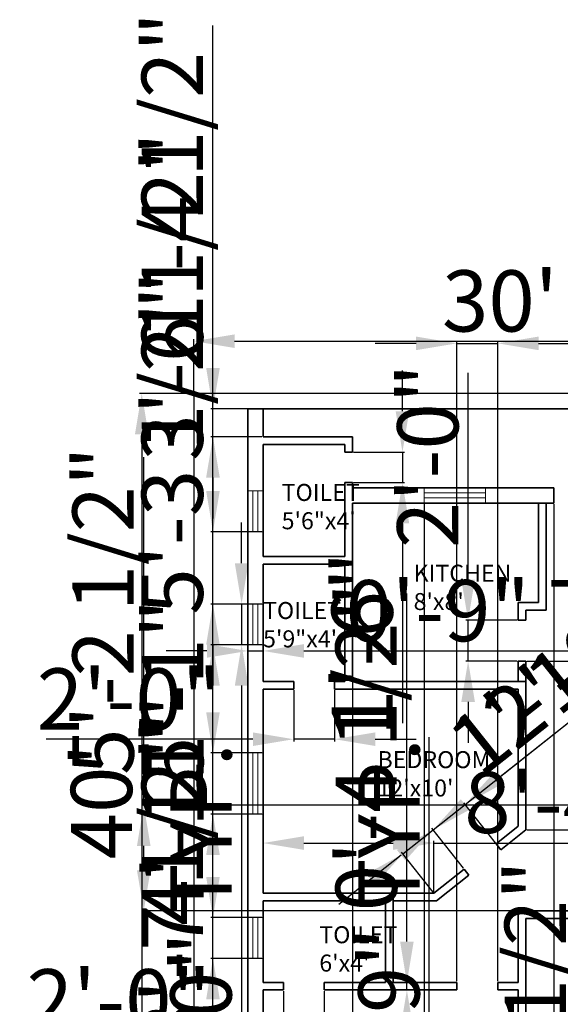
# Model space of a CAD drawing. Units: inches. Extents: x 1041 to 1781, y -140 to 732.
# Tile 2 of 6: x 1041 to 1359, y 153 to 732. Entities that reach past the tile are written whole.
import ezdxf

# ---------------------------------------------------------------- set-up
doc = ezdxf.new("R2010")
doc.units = ezdxf.units.IN
for name, color, linetype, lineweight in [('A-AREA-IDEN', 7, 'Continuous', 20), ('A-GLAZ', 4, 'Continuous', 18), ('A-WALL', 7, 'Continuous', 35), ('C-PROP', 3, 'Continuous', 25), ('dimension', 130, 'Continuous', 18)]:
    doc.layers.add(name, color=color, linetype=linetype, lineweight=lineweight)
doc.styles.get("Standard").update_dxf_attribs({"font": 'arial.ttf'})
doc.dimstyles.new('ISO-25', dxfattribs={"dimtxt": 36, "dimasz": 24, "dimexe": 1.25, "dimexo": 0.625, "dimtad": 1, "dimlunit": 4, "dimtxsty": 'Standard', "dimcen": 2.5, "dimadec": 0, "dimazin": 0, "dimtfac": 1, "dimtmove": 0, "dimatfit": 3, "dimfxl": 1, "dimarcsym": 0})

# ---------------------------------------------------------------- blocks, each defined once
blk = doc.blocks.new('*D1')
at = {"layer": 'Defpoints', "color": 0, "transparency": 16777216}
for p in [(1503.25, 542.96), (1143.25, 512.23), (1503.25, 512.23)]:
    blk.add_point(p, dxfattribs=at)
at = {"layer": 'dimension', "color": 0, "lineweight": -2, "transparency": 16777216}
for p, q in [((1143.25, 512.86), (1143.25, 544.21)), ((1167.25, 542.96), (1479.25, 542.96)), ((1503.25, 512.86), (1503.25, 544.21))]:
    blk.add_line(p, q, dxfattribs=at)
at = {"layer": 'dimension', "color": 0, "transparency": 16777216}
for points in [[(1167.25, 546.96), (1167.25, 538.96), (1143.25, 542.96)], [(1479.25, 546.96), (1479.25, 538.96), (1503.25, 542.96)]]:
    blk.add_solid(points, dxfattribs=at)
at = {"layer": 'dimension', "color": 0, "transparency": 16777216, "insert": (1323.25, 561.98), "char_height": 36, "attachment_point": 5}
blk.add_mtext("30'", dxfattribs=at)
blk = doc.blocks.new('*D2')
at = {"layer": 'Defpoints', "color": 0, "transparency": 16777216}
for p in [(1143.25, 512.23), (1112.63, 32.23), (1143.25, 32.23)]:
    blk.add_point(p, dxfattribs=at)
at = {"layer": 'dimension', "color": 0, "lineweight": -2, "transparency": 16777216}
for p, q in [((1142.62, 512.23), (1111.38, 512.23)), ((1112.63, 488.23), (1112.63, 56.23)), ((1142.62, 32.23), (1111.38, 32.23))]:
    blk.add_line(p, q, dxfattribs=at)
at = {"layer": 'dimension', "color": 0, "transparency": 16777216}
for points in [[(1108.63, 488.23), (1116.63, 488.23), (1112.63, 512.23)], [(1108.63, 56.23), (1116.63, 56.23), (1112.63, 32.23)]]:
    blk.add_solid(points, dxfattribs=at)
at = {"layer": 'dimension', "color": 0, "transparency": 16777216, "insert": (1093.62, 272.23), "char_height": 36, "attachment_point": 5, "rotation": 90}
blk.add_mtext("40'", dxfattribs=at)
blk = doc.blocks.new('WIN-36IN')
for p, q in [((0, 9), (0, 0)), ((36, 9), (0, 9)), ((36, 6), (0, 6)), ((36, 0), (36, 9)), ((0, 3), (36, 3)), ((0, 0), (36, 0)), ((0, 0), (36, 0))]:
    blk.add_line(p, q)
blk = doc.blocks.new('WIN-24IN')
for p, q in [((0, 9), (24, 9)), ((24, 9), (0, 9)), ((0, 9), (0, 0)), ((24, 6), (0, 6)), ((24, 0), (24, 9)), ((0, 3), (24, 3)), ((0, 0), (24, 0))]:
    blk.add_line(p, q)
blk = doc.blocks.new('*D9')
at = {"layer": 'Defpoints', "color": 0, "transparency": 16777216}
for p in [(1174.94, 388.32), (1171.34, 364.32), (1174.94, 364.32)]:
    blk.add_point(p, dxfattribs=at)
at = {"layer": 'dimension', "color": 0, "lineweight": -2, "transparency": 16777216}
for p, q in [((1171.34, 412.32), (1171.34, 436.32)), ((1174.31, 388.32), (1170.09, 388.32)), ((1171.34, 388.32), (1171.34, 364.32)), ((1174.31, 364.32), (1170.09, 364.32)), ((1171.34, 340.32), (1171.34, -140.48))]:
    blk.add_line(p, q, dxfattribs=at)
at = {"layer": 'dimension', "color": 0, "transparency": 16777216}
for points in [[(1167.34, 412.32), (1175.34, 412.32), (1171.34, 388.32)], [(1167.34, 340.32), (1175.34, 340.32), (1171.34, 364.32)]]:
    blk.add_solid(points, dxfattribs=at)
at = {"layer": 'dimension', "color": 0, "transparency": 16777216, "insert": (1152.09, 87.92), "char_height": 36, "attachment_point": 5, "rotation": 90}
blk.add_mtext('WINDOW 2\'-0" TYP.', dxfattribs=at)
blk = doc.blocks.new('*D10')
at = {"layer": 'Defpoints', "color": 0, "transparency": 16777216}
for p in [(1174.94, 364.32), (1183.94, 364.32), (1183.94, 360.72)]:
    blk.add_point(p, dxfattribs=at)
at = {"layer": 'dimension', "color": 0, "lineweight": -2, "transparency": 16777216}
for p, q in [((1150.94, 360.72), (1126.94, 360.72)), ((1174.94, 363.69), (1174.94, 359.47)), ((1174.94, 360.72), (1183.94, 360.72)), ((1183.94, 363.69), (1183.94, 359.47)), ((1207.94, 360.72), (1452.63, 360.72))]:
    blk.add_line(p, q, dxfattribs=at)
at = {"layer": 'dimension', "color": 0, "transparency": 16777216}
for points in [[(1150.94, 364.72), (1150.94, 356.72), (1174.94, 360.72)], [(1207.94, 364.72), (1207.94, 356.72), (1183.94, 360.72)]]:
    blk.add_solid(points, dxfattribs=at)
at = {"layer": 'dimension', "color": 0, "transparency": 16777216, "insert": (1342.28, 379.72), "char_height": 36, "attachment_point": 5}
blk.add_mtext('0\'-9" TYP.', dxfattribs=at)
blk = doc.blocks.new('*D12')
at = {"layer": 'Defpoints', "color": 0, "transparency": 16777216}
for p in [(1276.2, 41.23), (1281.6, 41.23), (1276.2, 32.23)]:
    blk.add_point(p, dxfattribs=at)
at = {"layer": 'dimension', "color": 0, "lineweight": -2, "transparency": 16777216}
for p, q in [((1281.6, 65.23), (1281.6, 309.92)), ((1276.83, 41.23), (1282.85, 41.23)), ((1281.6, 32.23), (1281.6, 41.23)), ((1276.83, 32.23), (1282.85, 32.23)), ((1281.6, 8.23), (1281.6, -15.77))]:
    blk.add_line(p, q, dxfattribs=at)
at = {"layer": 'dimension', "color": 0, "transparency": 16777216}
for points in [[(1277.6, 65.23), (1285.6, 65.23), (1281.6, 41.23)], [(1277.6, 8.23), (1285.6, 8.23), (1281.6, 32.23)]]:
    blk.add_solid(points, dxfattribs=at)
at = {"layer": 'dimension', "color": 0, "transparency": 16777216, "insert": (1262.59, 199.58), "char_height": 36, "attachment_point": 5, "rotation": 90}
blk.add_mtext('0\'-9" TYP.', dxfattribs=at)
blk = doc.blocks.new('*D19')
at = {"layer": 'Defpoints', "color": 0, "transparency": 16777216}
for p in [(1354.94, 447.73), (1390.94, 447.73), (1390.94, 2.78)]:
    blk.add_point(p, dxfattribs=at)
at = {"layer": 'dimension', "color": 0, "lineweight": -2, "transparency": 16777216}
for p, q in [((1354.94, 447.11), (1354.94, 1.53)), ((1390.94, 447.11), (1390.94, 1.53)), ((1330.94, 2.78), (1306.94, 2.78)), ((1354.94, 2.78), (1390.94, 2.78)), ((1414.94, 2.78), (1535.86, 2.78))]:
    blk.add_line(p, q, dxfattribs=at)
at = {"layer": 'dimension', "color": 0, "transparency": 16777216}
for points in [[(1330.94, 6.78), (1330.94, -1.22), (1354.94, 2.78)], [(1414.94, 6.78), (1414.94, -1.22), (1390.94, 2.78)]]:
    blk.add_solid(points, dxfattribs=at)
at = {"layer": 'dimension', "color": 0, "transparency": 16777216, "insert": (1487.4, 21.8), "char_height": 36, "attachment_point": 5}
blk.add_mtext('3\'-0"', dxfattribs=at)
blk = doc.blocks.new('*D23')
at = {"layer": 'Defpoints', "color": 0, "transparency": 16777216}
for p in [(1302.68, 270.36), (1321, 247.3), (1302.2, 232.37)]:
    blk.add_point(p, dxfattribs=at)
at = {"layer": 'dimension', "color": 0, "lineweight": -2, "transparency": 16777216}
for p, q in [((1321.47, 285.29), (1416.66, 360.9)), ((1283.89, 255.44), (1302.68, 270.36)), ((1320.61, 247.79), (1301.9, 271.34)), ((1301.82, 232.86), (1283.11, 256.41)), ((1265.09, 240.51), (1246.3, 225.58))]:
    blk.add_line(p, q, dxfattribs=at)
at = {"layer": 'dimension', "color": 0, "transparency": 16777216}
for points in [[(1318.99, 288.42), (1323.96, 282.16), (1302.68, 270.36)], [(1262.61, 243.64), (1267.58, 237.38), (1283.89, 255.44)]]:
    blk.add_solid(points, dxfattribs=at)
at = {"layer": 'dimension', "color": 0, "transparency": 16777216, "insert": (1366.64, 345.44), "char_height": 36, "attachment_point": 5, "rotation": 38.45936}
blk.add_mtext('2\'-0"', dxfattribs=at)
blk = doc.blocks.new('*D24')
at = {"layer": 'Defpoints', "color": 0, "transparency": 16777216}
for p in [(1154.49, 84.57), (1183.94, 84.57), (1183.94, 41.23)]:
    blk.add_point(p, dxfattribs=at)
at = {"layer": 'dimension', "color": 0, "lineweight": -2, "transparency": 16777216}
for p, q in [((1154.49, 108.57), (1154.49, 313.38)), ((1183.31, 84.57), (1153.24, 84.57)), ((1154.49, 41.23), (1154.49, 84.57)), ((1183.31, 41.23), (1153.24, 41.23)), ((1154.49, 17.23), (1154.49, -6.77))]:
    blk.add_line(p, q, dxfattribs=at)
at = {"layer": 'dimension', "color": 0, "transparency": 16777216}
for points in [[(1150.49, 108.57), (1158.49, 108.57), (1154.49, 84.57)], [(1150.49, 17.23), (1158.49, 17.23), (1154.49, 41.23)]]:
    blk.add_solid(points, dxfattribs=at)
at = {"layer": 'dimension', "color": 0, "transparency": 16777216, "insert": (1135.24, 222.98), "char_height": 36, "attachment_point": 5, "rotation": 90}
blk.add_mtext('3\'-7 1/2"', dxfattribs=at)
blk = doc.blocks.new('*D25')
at = {"layer": 'Defpoints', "color": 0, "transparency": 16777216}
for p in [(1154.49, 179.79), (1183.94, 179.79), (1183.94, 120.57)]:
    blk.add_point(p, dxfattribs=at)
at = {"layer": 'dimension', "color": 0, "lineweight": -2, "transparency": 16777216}
for p, q in [((1154.49, 179.79), (1154.49, 330.15)), ((1183.31, 179.79), (1153.24, 179.79)), ((1154.49, 144.57), (1154.49, 155.79)), ((1183.31, 120.57), (1153.24, 120.57))]:
    blk.add_line(p, q, dxfattribs=at)
at = {"layer": 'dimension', "color": 0, "transparency": 16777216}
for points in [[(1150.49, 155.79), (1158.49, 155.79), (1154.49, 179.79)], [(1150.49, 144.57), (1158.49, 144.57), (1154.49, 120.57)]]:
    blk.add_solid(points, dxfattribs=at)
at = {"layer": 'dimension', "color": 0, "transparency": 16777216, "insert": (1135.79, 266.97), "char_height": 36, "attachment_point": 5, "rotation": 90}
blk.add_mtext('4\'-11"', dxfattribs=at)
blk = doc.blocks.new('*D26')
at = {"layer": 'Defpoints', "color": 0, "transparency": 16777216}
for p in [(1154.49, 264.67), (1183.94, 264.67), (1183.94, 203.79)]:
    blk.add_point(p, dxfattribs=at)
at = {"layer": 'dimension', "color": 0, "lineweight": -2, "transparency": 16777216}
for p, q in [((1154.49, 264.67), (1154.49, 385.62)), ((1183.31, 264.67), (1153.24, 264.67)), ((1154.49, 227.79), (1154.49, 240.67)), ((1183.31, 203.79), (1153.24, 203.79))]:
    blk.add_line(p, q, dxfattribs=at)
at = {"layer": 'dimension', "color": 0, "transparency": 16777216}
for points in [[(1150.49, 240.67), (1158.49, 240.67), (1154.49, 264.67)], [(1150.49, 227.79), (1158.49, 227.79), (1154.49, 203.79)]]:
    blk.add_solid(points, dxfattribs=at)
at = {"layer": 'dimension', "color": 0, "transparency": 16777216, "insert": (1135.48, 337.15), "char_height": 36, "attachment_point": 5, "rotation": 90}
blk.add_mtext('5\'-1"', dxfattribs=at)
blk = doc.blocks.new('*D27')
at = {"layer": 'Defpoints', "color": 0, "transparency": 16777216}
for p in [(1154.49, 364.32), (1183.94, 364.32), (1183.94, 300.67)]:
    blk.add_point(p, dxfattribs=at)
at = {"layer": 'dimension', "color": 0, "lineweight": -2, "transparency": 16777216}
for p, q in [((1154.49, 364.32), (1154.49, 569.15)), ((1183.31, 364.32), (1153.24, 364.32)), ((1154.49, 324.67), (1154.49, 340.32)), ((1183.31, 300.67), (1153.24, 300.67))]:
    blk.add_line(p, q, dxfattribs=at)
at = {"layer": 'dimension', "color": 0, "transparency": 16777216}
for points in [[(1150.49, 340.32), (1158.49, 340.32), (1154.49, 364.32)], [(1150.49, 324.67), (1158.49, 324.67), (1154.49, 300.67)]]:
    blk.add_solid(points, dxfattribs=at)
at = {"layer": 'dimension', "color": 0, "transparency": 16777216, "insert": (1135.24, 478.73), "char_height": 36, "attachment_point": 5, "rotation": 90}
blk.add_mtext('5\'-3 1/2"', dxfattribs=at)
blk = doc.blocks.new('*D28')
at = {"layer": 'Defpoints', "color": 0, "transparency": 16777216}
for p in [(1154.49, 430.87), (1183.94, 430.87), (1183.94, 388.32)]:
    blk.add_point(p, dxfattribs=at)
at = {"layer": 'dimension', "color": 0, "lineweight": -2, "transparency": 16777216}
for p, q in [((1154.49, 454.87), (1154.49, 659.68)), ((1183.31, 430.87), (1153.24, 430.87)), ((1154.49, 388.32), (1154.49, 430.87)), ((1183.31, 388.32), (1153.24, 388.32)), ((1154.49, 364.32), (1154.49, 340.32))]:
    blk.add_line(p, q, dxfattribs=at)
at = {"layer": 'dimension', "color": 0, "transparency": 16777216}
for points in [[(1150.49, 454.87), (1158.49, 454.87), (1154.49, 430.87)], [(1150.49, 364.32), (1158.49, 364.32), (1154.49, 388.32)]]:
    blk.add_solid(points, dxfattribs=at)
at = {"layer": 'dimension', "color": 0, "transparency": 16777216, "insert": (1135.24, 569.28), "char_height": 36, "attachment_point": 5, "rotation": 90}
blk.add_mtext('3\'-6 1/2"', dxfattribs=at)
blk = doc.blocks.new('*D29')
at = {"layer": 'Defpoints', "color": 0, "transparency": 16777216}
for p in [(1113.8, 269.99), (1467.44, 269.99), (1467.44, 207.73)]:
    blk.add_point(p, dxfattribs=at)
at = {"layer": 'dimension', "color": 0, "lineweight": -2, "transparency": 16777216}
for p, q in [((1113.8, 269.99), (1113.8, 474.82)), ((1466.81, 269.99), (1112.55, 269.99)), ((1113.8, 231.73), (1113.8, 245.99)), ((1466.81, 207.73), (1112.55, 207.73))]:
    blk.add_line(p, q, dxfattribs=at)
at = {"layer": 'dimension', "color": 0, "transparency": 16777216}
for points in [[(1109.8, 245.99), (1117.8, 245.99), (1113.8, 269.99)], [(1109.8, 231.73), (1117.8, 231.73), (1113.8, 207.73)]]:
    blk.add_solid(points, dxfattribs=at)
at = {"layer": 'dimension', "color": 0, "transparency": 16777216, "insert": (1094.56, 384.41), "char_height": 36, "attachment_point": 5, "rotation": 90}
blk.add_mtext('5\'-2 1/2"', dxfattribs=at)
blk = doc.blocks.new('*D31')
at = {"layer": 'Defpoints', "color": 0, "transparency": 16777216}
for p in [(1390.94, 447.73), (1427, 447.73), (1427, 2.78)]:
    blk.add_point(p, dxfattribs=at)
at = {"layer": 'dimension', "color": 0, "lineweight": -2, "transparency": 16777216}
for p, q in [((1390.94, 447.11), (1390.94, 1.53)), ((1427, 447.11), (1427, 1.53)), ((1366.94, 2.78), (1342.94, 2.78)), ((1390.94, 2.78), (1427, 2.78)), ((1451, 2.78), (1571.93, 2.78))]:
    blk.add_line(p, q, dxfattribs=at)
at = {"layer": 'dimension', "color": 0, "transparency": 16777216}
for points in [[(1366.94, 6.78), (1366.94, -1.22), (1390.94, 2.78)], [(1451, 6.78), (1451, -1.22), (1427, 2.78)]]:
    blk.add_solid(points, dxfattribs=at)
at = {"layer": 'dimension', "color": 0, "transparency": 16777216, "insert": (1523.46, 21.8), "char_height": 36, "attachment_point": 5}
blk.add_mtext('3\'-0"', dxfattribs=at)
blk = doc.blocks.new('*D32')
at = {"layer": 'Defpoints', "color": 0, "transparency": 16777216}
for p in [(1236.44, 447.73), (1278.74, 447.73), (1278.74, 2.78)]:
    blk.add_point(p, dxfattribs=at)
at = {"layer": 'dimension', "color": 0, "lineweight": -2, "transparency": 16777216}
for p, q in [((1236.44, 447.11), (1236.44, 1.53)), ((1278.74, 447.11), (1278.74, 1.53)), ((1212.44, 2.78), (1188.44, 2.78)), ((1236.44, 2.78), (1278.74, 2.78)), ((1302.74, 2.78), (1507.55, 2.78))]:
    blk.add_line(p, q, dxfattribs=at)
at = {"layer": 'dimension', "color": 0, "transparency": 16777216}
for points in [[(1212.44, 6.78), (1212.44, -1.22), (1236.44, 2.78)], [(1302.74, 6.78), (1302.74, -1.22), (1278.74, 2.78)]]:
    blk.add_solid(points, dxfattribs=at)
at = {"layer": 'dimension', "color": 0, "transparency": 16777216, "insert": (1417.15, 22.03), "char_height": 36, "attachment_point": 5}
blk.add_mtext('3\'-6 1/2"', dxfattribs=at)
blk = doc.blocks.new('*D34')
at = {"layer": 'Defpoints', "color": 0, "transparency": 16777216}
for p in [(1236.44, 477.73), (1236.44, 459.73), (1265.89, 459.73)]:
    blk.add_point(p, dxfattribs=at)
at = {"layer": 'dimension', "color": 0, "lineweight": -2, "transparency": 16777216}
for p, q in [((1265.89, 501.73), (1265.89, 525.73)), ((1237.06, 477.73), (1267.14, 477.73)), ((1265.89, 477.73), (1265.89, 459.73)), ((1237.06, 459.73), (1267.14, 459.73)), ((1265.89, 435.73), (1265.89, 318.17))]:
    blk.add_line(p, q, dxfattribs=at)
at = {"layer": 'dimension', "color": 0, "transparency": 16777216}
for points in [[(1261.89, 501.73), (1269.89, 501.73), (1265.89, 477.73)], [(1261.89, 435.73), (1269.89, 435.73), (1265.89, 459.73)]]:
    blk.add_solid(points, dxfattribs=at)
at = {"layer": 'dimension', "color": 0, "transparency": 16777216, "insert": (1246.88, 364.95), "char_height": 36, "attachment_point": 5, "rotation": 90}
blk.add_mtext('1\'-6"', dxfattribs=at)
blk = doc.blocks.new('*D35')
at = {"layer": 'Defpoints', "color": 0, "transparency": 16777216}
for p in [(1321.94, 541.68), (1297.94, 165.73), (1321.94, 165.73)]:
    blk.add_point(p, dxfattribs=at)
at = {"layer": 'dimension', "color": 0, "lineweight": -2, "transparency": 16777216}
for p, q in [((1273.94, 541.68), (1249.94, 541.68)), ((1297.94, 166.36), (1297.94, 542.93)), ((1297.94, 541.68), (1321.94, 541.68)), ((1321.94, 166.36), (1321.94, 542.93)), ((1345.94, 541.68), (1467.5, 541.68))]:
    blk.add_line(p, q, dxfattribs=at)
at = {"layer": 'dimension', "color": 0, "transparency": 16777216}
for points in [[(1273.94, 545.68), (1273.94, 537.68), (1297.94, 541.68)], [(1345.94, 545.68), (1345.94, 537.68), (1321.94, 541.68)]]:
    blk.add_solid(points, dxfattribs=at)
at = {"layer": 'dimension', "color": 0, "transparency": 16777216, "insert": (1418.72, 560.69), "char_height": 36, "attachment_point": 5}
blk.add_mtext('2\'-0"', dxfattribs=at)
blk = doc.blocks.new('*D36')
at = {"layer": 'Defpoints', "color": 0, "transparency": 16777216}
for p in [(1195.94, 161.23), (1219.94, 161.23), (1195.94, 131.78)]:
    blk.add_point(p, dxfattribs=at)
at = {"layer": 'dimension', "color": 0, "lineweight": -2, "transparency": 16777216}
for p, q in [((1195.94, 160.61), (1195.94, 130.53)), ((1219.94, 160.61), (1219.94, 130.53)), ((1171.94, 131.78), (1050.38, 131.78)), ((1219.94, 131.78), (1195.94, 131.78)), ((1243.94, 131.78), (1267.94, 131.78))]:
    blk.add_line(p, q, dxfattribs=at)
at = {"layer": 'dimension', "color": 0, "transparency": 16777216}
for points in [[(1171.94, 135.78), (1171.94, 127.78), (1195.94, 131.78)], [(1243.94, 135.78), (1243.94, 127.78), (1219.94, 131.78)]]:
    blk.add_solid(points, dxfattribs=at)
at = {"layer": 'dimension', "color": 0, "transparency": 16777216, "insert": (1099.16, 150.79), "char_height": 36, "attachment_point": 5}
blk.add_mtext('2\'-0"', dxfattribs=at)
blk = doc.blocks.new('*D37')
at = {"layer": 'Defpoints', "color": 0, "transparency": 16777216}
for p in [(1201.94, 338.23), (1225.94, 338.23), (1201.94, 308.78)]:
    blk.add_point(p, dxfattribs=at)
at = {"layer": 'dimension', "color": 0, "lineweight": -2, "transparency": 16777216}
for p, q in [((1201.94, 337.61), (1201.94, 307.53)), ((1225.94, 337.61), (1225.94, 307.53)), ((1177.94, 308.78), (1056.38, 308.78)), ((1225.94, 308.78), (1201.94, 308.78)), ((1249.94, 308.78), (1273.94, 308.78))]:
    blk.add_line(p, q, dxfattribs=at)
at = {"layer": 'dimension', "color": 0, "transparency": 16777216}
for points in [[(1177.94, 312.78), (1177.94, 304.78), (1201.94, 308.78)], [(1249.94, 312.78), (1249.94, 304.78), (1225.94, 308.78)]]:
    blk.add_solid(points, dxfattribs=at)
at = {"layer": 'dimension', "color": 0, "transparency": 16777216, "insert": (1105.16, 327.79), "char_height": 36, "attachment_point": 5}
blk.add_mtext('2\'-0"', dxfattribs=at)
blk = doc.blocks.new('*D38')
at = {"layer": 'Defpoints', "color": 0, "transparency": 16777216}
for p in [(1304.49, 378.73), (1333.94, 378.73), (1333.94, 354.73)]:
    blk.add_point(p, dxfattribs=at)
at = {"layer": 'dimension', "color": 0, "lineweight": -2, "transparency": 16777216}
for p, q in [((1304.49, 402.73), (1304.49, 524.29)), ((1333.31, 378.73), (1303.24, 378.73)), ((1304.49, 354.73), (1304.49, 378.73)), ((1333.31, 354.73), (1303.24, 354.73)), ((1304.49, 330.73), (1304.49, 306.73))]:
    blk.add_line(p, q, dxfattribs=at)
at = {"layer": 'dimension', "color": 0, "transparency": 16777216}
for points in [[(1300.49, 402.73), (1308.49, 402.73), (1304.49, 378.73)], [(1300.49, 330.73), (1308.49, 330.73), (1304.49, 354.73)]]:
    blk.add_solid(points, dxfattribs=at)
at = {"layer": 'dimension', "color": 0, "transparency": 16777216, "insert": (1285.48, 475.51), "char_height": 36, "attachment_point": 5, "rotation": 90}
blk.add_mtext('2\'-0"', dxfattribs=at)
blk = doc.blocks.new('*D40')
at = {"layer": 'Defpoints', "color": 0, "transparency": 16777216}
for p in [(1154.49, 503.23), (1183.94, 503.23), (1183.94, 486.73)]:
    blk.add_point(p, dxfattribs=at)
at = {"layer": 'dimension', "color": 0, "lineweight": -2, "transparency": 16777216}
for p, q in [((1154.49, 527.23), (1154.49, 728.68)), ((1183.31, 503.23), (1153.24, 503.23)), ((1154.49, 486.73), (1154.49, 503.23)), ((1183.31, 486.73), (1153.24, 486.73)), ((1154.49, 462.73), (1154.49, 438.73))]:
    blk.add_line(p, q, dxfattribs=at)
at = {"layer": 'dimension', "color": 0, "transparency": 16777216}
for points in [[(1150.49, 527.23), (1158.49, 527.23), (1154.49, 503.23)], [(1150.49, 462.73), (1158.49, 462.73), (1154.49, 486.73)]]:
    blk.add_solid(points, dxfattribs=at)
at = {"layer": 'dimension', "color": 0, "transparency": 16777216, "insert": (1135.25, 639.95), "char_height": 36, "attachment_point": 5, "rotation": 90}
blk.add_mtext('1\'-4 1/2"', dxfattribs=at)
blk = doc.blocks.new('*D41')
at = {"layer": 'Defpoints', "color": 0, "transparency": 16777216}
for p in [(1268.49, 165.73), (1297.94, 165.73), (1297.94, 161.23)]:
    blk.add_point(p, dxfattribs=at)
at = {"layer": 'dimension', "color": 0, "lineweight": -2, "transparency": 16777216}
for p, q in [((1268.49, 189.73), (1268.49, 394.57)), ((1297.31, 165.73), (1267.24, 165.73)), ((1268.49, 161.23), (1268.49, 165.73)), ((1297.31, 161.23), (1267.24, 161.23)), ((1268.49, 137.23), (1268.49, 113.23))]:
    blk.add_line(p, q, dxfattribs=at)
at = {"layer": 'dimension', "color": 0, "transparency": 16777216}
for points in [[(1264.49, 189.73), (1272.49, 189.73), (1268.49, 165.73)], [(1264.49, 137.23), (1272.49, 137.23), (1268.49, 161.23)]]:
    blk.add_solid(points, dxfattribs=at)
at = {"layer": 'dimension', "color": 0, "transparency": 16777216, "insert": (1249.25, 304.15), "char_height": 36, "attachment_point": 5, "rotation": 90}
blk.add_mtext('0\'-4 1/2"', dxfattribs=at)
blk = doc.blocks.new('*D43')
at = {"layer": 'Defpoints', "color": 0, "transparency": 16777216}
for p in [(1284.4, 247.68), (1183.94, 218.23), (1284.4, 218.23)]:
    blk.add_point(p, dxfattribs=at)
at = {"layer": 'dimension', "color": 0, "lineweight": -2, "transparency": 16777216}
for p, q in [((1183.94, 218.86), (1183.94, 248.93)), ((1207.94, 247.68), (1260.4, 247.68)), ((1284.4, 218.86), (1284.4, 248.93)), ((1284.4, 247.68), (1489.28, 247.68))]:
    blk.add_line(p, q, dxfattribs=at)
at = {"layer": 'dimension', "color": 0, "transparency": 16777216}
for points in [[(1207.94, 251.68), (1207.94, 243.68), (1183.94, 247.68)], [(1260.4, 251.68), (1260.4, 243.68), (1284.4, 247.68)]]:
    blk.add_solid(points, dxfattribs=at)
at = {"layer": 'dimension', "color": 0, "transparency": 16777216, "insert": (1398.84, 266.92), "char_height": 36, "attachment_point": 5}
blk.add_mtext('8\'-4 1/2"', dxfattribs=at)
blk = doc.blocks.new('*D44')
at = {"layer": 'Defpoints', "color": 0, "transparency": 16777216}
for p in [(1338.44, 354.73), (1338.44, 255.41), (1367.89, 255.41)]:
    blk.add_point(p, dxfattribs=at)
at = {"layer": 'dimension', "color": 0, "lineweight": -2, "transparency": 16777216}
for p, q in [((1339.06, 354.73), (1369.14, 354.73)), ((1367.89, 330.73), (1367.89, 279.41)), ((1339.06, 255.41), (1369.14, 255.41)), ((1367.89, 255.41), (1367.89, 50.53))]:
    blk.add_line(p, q, dxfattribs=at)
at = {"layer": 'dimension', "color": 0, "transparency": 16777216}
for points in [[(1363.89, 330.73), (1371.89, 330.73), (1367.89, 354.73)], [(1363.89, 279.41), (1371.89, 279.41), (1367.89, 255.41)]]:
    blk.add_solid(points, dxfattribs=at)
at = {"layer": 'dimension', "color": 0, "transparency": 16777216, "insert": (1348.64, 140.97), "char_height": 36, "attachment_point": 5, "rotation": 90}
blk.add_mtext('8\'-3 1/2"', dxfattribs=at)
blk = doc.blocks.new('*D45')
at = {"layer": 'Defpoints', "color": 0, "transparency": 16777216}
for p in [(1283.89, 255.44), (1302.2, 232.37), (1284.4, 218.23)]:
    blk.add_point(p, dxfattribs=at)
at = {"layer": 'dimension', "color": 0, "lineweight": -2, "transparency": 16777216}
for p, q in [((1302.68, 270.36), (1482.32, 413.05)), ((1266.08, 241.29), (1283.89, 255.44)), ((1301.82, 232.86), (1283.11, 256.41)), ((1284.01, 218.72), (1265.3, 242.27)), ((1247.29, 226.37), (1228.5, 211.44))]:
    blk.add_line(p, q, dxfattribs=at)
at = {"layer": 'dimension', "color": 0, "transparency": 16777216}
for points in [[(1300.19, 273.49), (1305.17, 267.23), (1283.89, 255.44)], [(1244.8, 229.5), (1249.78, 223.23), (1266.08, 241.29)]]:
    blk.add_solid(points, dxfattribs=at)
at = {"layer": 'dimension', "color": 0, "transparency": 16777216, "insert": (1389.93, 364.23), "char_height": 36, "attachment_point": 5, "rotation": 38.45936}
blk.add_mtext('1\'-10 1/2"', dxfattribs=at)

msp = doc.modelspace()

# ---------------------------------------------------------------- linework, layer by layer
at = {"layer": 'A-GLAZ'}
for p, q in [((1278.743, 456.733), (1278.743, 447.733)), ((1278.743, 456.733), (1314.743, 456.733)), ((1314.743, 453.733), (1278.743, 453.733)), ((1314.743, 447.733), (1314.743, 456.733)), ((1278.743, 450.733), (1314.743, 450.733)), ((1278.743, 447.733), (1314.743, 447.733))]:
    msp.add_line(p, q, dxfattribs=at)
at = {"layer": 'A-WALL'}
for p, q in [((1498.749, 503.233), (1174.938, 503.233)), ((1174.938, 41.233), (1174.938, 503.233)), ((1183.938, 486.733), (1183.938, 503.233)), ((1183.938, 486.733), (1236.438, 486.733)), ((1231.938, 486.733), (1236.438, 486.733)), ((1236.438, 477.733), (1236.438, 486.733)), ((1183.938, 482.233), (1231.938, 482.233)), ((1183.938, 416.233), (1183.938, 482.233)), ((1231.938, 477.733), (1231.938, 482.233)), ((1231.938, 477.733), (1236.438, 477.733)), ((1231.938, 416.233), (1231.938, 459.733)), ((1231.938, 459.733), (1236.438, 459.733)), ((1236.438, 456.733), (1236.438, 459.733)), ((1236.438, 456.733), (1354.938, 456.733)), ((1354.938, 447.733), (1354.938, 456.733)), ((1236.438, 447.733), (1354.938, 447.733)), ((1236.438, 342.733), (1236.438, 447.733)), ((1345.938, 389.233), (1345.938, 447.733)), ((1350.438, 384.733), (1350.438, 447.733)), ((1183.938, 416.233), (1231.938, 416.233)), ((1183.938, 411.733), (1231.938, 411.733)), ((1183.938, 342.733), (1183.938, 411.733)), ((1231.938, 342.733), (1231.938, 411.733)), ((1333.938, 378.733), (1333.938, 389.233)), ((1333.938, 389.233), (1345.938, 389.233)), ((1338.438, 378.733), (1338.438, 384.733)), ((1338.438, 384.733), (1350.438, 384.733)), ((1333.938, 378.733), (1338.438, 378.733)), ((1333.938, 342.733), (1333.938, 354.733)), ((1333.938, 354.733), (1338.438, 354.733)), ((1338.438, 255.408), (1338.438, 354.733)), ((1183.938, 342.733), (1201.938, 342.733)), ((1201.938, 338.233), (1201.938, 342.733)), ((1225.938, 338.233), (1225.938, 342.733)), ((1225.938, 342.733), (1231.938, 342.733)), ((1236.438, 342.733), (1338.438, 342.733)), ((1183.938, 338.233), (1201.938, 338.233)), ((1183.938, 218.233), (1183.938, 338.233)), ((1225.938, 338.233), (1333.938, 338.233)), ((1333.938, 257.58), (1333.938, 338.233)), ((1333.938, 257.58), (1320.997, 247.302)), ((1338.438, 255.408), (1323.796, 243.778)), ((1320.997, 247.302), (1323.796, 243.778)), ((1302.204, 232.375), (1284.399, 218.233)), ((1302.204, 232.375), (1305.003, 228.851)), ((1305.003, 228.851), (1285.968, 213.733)), ((1183.938, 218.233), (1284.399, 218.233)), ((1260.438, 165.733), (1260.438, 218.233)), ((1183.938, 213.733), (1255.938, 213.733)), ((1183.938, 165.733), (1183.938, 213.733)), ((1255.938, 165.733), (1255.938, 213.733)), ((1260.438, 213.733), (1285.968, 213.733)), ((1333.938, 207.733), (1413.438, 207.733)), ((1333.938, 165.733), (1333.938, 207.733)), ((1338.438, 41.233), (1338.438, 203.233)), ((1338.438, 203.233), (1413.438, 203.233)), ((1183.938, 165.733), (1195.938, 165.733)), ((1183.938, 165.733), (1195.938, 165.733)), ((1195.938, 165.733), (1195.938, 161.233)), ((1219.938, 165.733), (1219.938, 161.233)), ((1219.938, 165.733), (1255.938, 165.733)), ((1260.438, 165.733), (1297.938, 165.733)), ((1297.938, 165.733), (1297.938, 161.233)), ((1333.938, 165.733), (1321.938, 165.733)), ((1321.938, 165.733), (1321.938, 161.233)), ((1321.938, 165.733), (1333.938, 165.733)), ((1183.938, 161.233), (1195.938, 161.233)), ((1183.938, 41.233), (1183.938, 161.233)), ((1219.938, 161.233), (1297.938, 161.233)), ((1321.938, 161.233), (1333.938, 161.233)), ((1333.938, 41.233), (1333.938, 161.233))]:
    msp.add_line(p, q, dxfattribs=at)
at = {"layer": 'C-PROP'}
for p, q in [((1503.249, 512.233), (1143.249, 512.233)), ((1143.249, 512.233), (1143.249, 32.233))]:
    msp.add_line(p, q, dxfattribs=at)

# ---------------------------------------------------------------- block references
at = {"layer": 'A-GLAZ'}
for name, p, rotation in [('WIN-24IN', (1174.938, 454.873), 269.9999999999987), ('WIN-24IN', (1174.938, 388.318), 269.9999999999987), ('WIN-36IN', (1183.937, 264.674), 89.9999999999994), ('WIN-24IN', (1174.938, 203.788), 269.9999999999986)]:
    msp.add_blockref(name, p, dxfattribs=dict(at, rotation=rotation))

# ---------------------------------------------------------------- texts
at = {"layer": 'A-AREA-IDEN', "char_height": 10, "attachment_point": 1}
for s, insert in [('TOILET\\P5\'6"x4\'', (1194.873, 458.97)), ("KITCHEN\\P8'x8'", (1272.445, 411.441)), ('TOILET\\P5\'9"x4\'', (1183.938, 389.504)), ("BEDROOM\\P12'x10'", (1251.223, 301.757)), ("TOILET\\P6'x4'", (1217.009, 198.743))]:
    msp.add_mtext_dynamic_manual_height_columns(s, width=64.5482, gutter_width=12.5, heights=[0], dxfattribs=dict(at, insert=insert))

# ---------------------------------------------------------------- dimensions: what is measured, and where the dimension line sits
at = {"layer": 'dimension'}
for base, p1, p2, angle, override, picture, middle in [((1154.488, 503.233), (1183.938, 486.733), (1183.938, 503.233), 90, {"dimdec": 1, "dimlfac": 1, "dimrnd": 0, "dimzin": 1, "dimdsep": 46, "dimlunit": 4, "dimfrac": 2}, '*D40', (1135.249, 639.954)), ((1154.488, 430.873), (1183.938, 388.318), (1183.938, 430.873), 90, {"dimdec": 1, "dimlfac": 1, "dimrnd": 0, "dimzin": 1, "dimdsep": 46, "dimlunit": 4, "dimfrac": 2}, '*D28', (1135.236, 569.277)), ((1154.488, 364.318), (1183.938, 300.673), (1183.938, 364.318), 90, {"dimdec": 1, "dimlfac": 1, "dimrnd": 0, "dimzin": 1, "dimdsep": 46, "dimlunit": 4, "dimfrac": 2}, '*D27', (1135.236, 478.734)), ((1304.488, 378.733), (1333.938, 354.733), (1333.938, 378.733), 90, {"dimdec": 1, "dimlfac": 1, "dimrnd": 0, "dimzin": 1, "dimdsep": 46, "dimlunit": 4, "dimfrac": 2}, '*D38', (1285.482, 475.513)), ((1265.888, 459.733), (1236.438, 477.733), (1236.438, 459.733), 270, {"dimdec": 1, "dimlfac": 1, "dimrnd": 0, "dimzin": 1, "dimdsep": 46, "dimlunit": 4, "dimfrac": 2}, '*D34', (1246.882, 364.953)), ((1112.63, 32.233), (1143.249, 512.233), (1143.249, 32.233), 90, {"dimclrd": 0, "dimclre": 0, "dimclrt": 0}, '*D2', (1093.625, 272.233)), ((1113.799, 269.99), (1467.438, 207.733), (1467.438, 269.99), 90, {"dimdec": 1, "dimlfac": 1, "dimrnd": 0, "dimzin": 1, "dimdsep": 46, "dimlunit": 4, "dimfrac": 2}, '*D29', (1094.56, 384.406)), ((1283.887, 255.436), (1284.399, 218.233), (1302.204, 232.375), 38.459364, {"dimdec": 1, "dimlfac": 1, "dimrnd": 0, "dimzin": 1, "dimdsep": 46, "dimlunit": 4, "dimfrac": 2}, '*D45', (1389.932, 364.234)), ((1268.488, 165.733), (1297.938, 161.233), (1297.938, 165.733), 90, {"dimdec": 1, "dimlfac": 1, "dimrnd": 0, "dimzin": 1, "dimdsep": 46, "dimlunit": 4, "dimfrac": 2}, '*D41', (1249.249, 304.149)), ((1302.68, 270.363), (1302.204, 232.375), (1320.997, 247.302), 38.459364, {"dimdec": 1, "dimlfac": 1, "dimrnd": 0, "dimzin": 1, "dimdsep": 46, "dimlunit": 4, "dimfrac": 2}, '*D23', (1366.644, 345.439)), ((1154.488, 264.673), (1183.938, 203.788), (1183.938, 264.673), 90, {"dimdec": 1, "dimlfac": 1, "dimrnd": 0, "dimzin": 1, "dimdsep": 46, "dimlunit": 4, "dimfrac": 2}, '*D26', (1135.482, 337.147)), ((1367.888, 255.408), (1338.438, 354.733), (1338.438, 255.408), 270, {"dimdec": 1, "dimlfac": 1, "dimrnd": 0, "dimzin": 1, "dimdsep": 46, "dimlunit": 4, "dimfrac": 2}, '*D44', (1348.636, 140.967)), ((1201.938, 308.783), (1225.938, 338.233), (1201.938, 338.233), 180, {"dimdec": 1, "dimlfac": 1, "dimrnd": 0, "dimzin": 1, "dimdsep": 46, "dimlunit": 4, "dimfrac": 2}, '*D37', (1105.157, 327.788)), ((1154.488, 179.788), (1183.938, 120.573), (1183.938, 179.788), 90, {"dimdec": 1, "dimlfac": 1, "dimrnd": 0, "dimzin": 1, "dimdsep": 46, "dimlunit": 4, "dimfrac": 2}, '*D25', (1135.789, 266.971)), ((1154.488, 84.573), (1183.938, 41.233), (1183.938, 84.573), 90, {"dimdec": 1, "dimlfac": 1, "dimrnd": 0, "dimzin": 1, "dimdsep": 46, "dimlunit": 4, "dimfrac": 2}, '*D24', (1135.236, 222.977)), ((1195.938, 131.783), (1219.938, 161.233), (1195.938, 161.233), 180, {"dimdec": 1, "dimlfac": 1, "dimrnd": 0, "dimzin": 1, "dimdsep": 46, "dimlunit": 4, "dimfrac": 2}, '*D36', (1099.157, 150.788))]:
    dim = msp.add_linear_dim(base=base, p1=p1, p2=p2, angle=angle, dimstyle='ISO-25', override=override, dxfattribs=at)
    dim.commit()
    dim.dimension.update_dxf_attribs({"geometry": picture, "text_midpoint": middle})
for base, p1, p2, override, picture, middle in [((1503.249, 542.957), (1143.249, 512.233), (1503.249, 512.233), {"dimclrd": 0, "dimclre": 0, "dimclrt": 0}, '*D1', (1323.249, 561.975)), ((1321.938, 541.683), (1297.938, 165.733), (1321.938, 165.733), {"dimdec": 1, "dimlfac": 1, "dimrnd": 0, "dimzin": 1, "dimdsep": 46, "dimlunit": 4, "dimfrac": 2}, '*D35', (1418.718, 560.688)), ((1278.743, 2.783), (1236.438, 447.733), (1278.743, 447.733), {"dimdec": 1, "dimlfac": 1, "dimrnd": 0, "dimzin": 1, "dimdsep": 46, "dimlunit": 4, "dimfrac": 2}, '*D32', (1417.147, 22.034)), ((1390.938, 2.783), (1354.938, 447.733), (1390.938, 447.733), {"dimdec": 1, "dimlfac": 1, "dimrnd": 0, "dimzin": 1, "dimdsep": 46, "dimlunit": 4, "dimfrac": 2}, '*D19', (1487.399, 21.8)), ((1427.003, 2.783), (1390.938, 447.733), (1427.003, 447.733), {"dimdec": 1, "dimlfac": 1, "dimrnd": 0, "dimzin": 1, "dimdsep": 46, "dimlunit": 4, "dimfrac": 2}, '*D31', (1523.464, 21.8)), ((1284.399, 247.683), (1183.938, 218.233), (1284.399, 218.233), {"dimdec": 1, "dimlfac": 1, "dimrnd": 0, "dimzin": 1, "dimdsep": 46, "dimlunit": 4, "dimfrac": 2}, '*D43', (1398.839, 266.921))]:
    dim = msp.add_linear_dim(base=base, p1=p1, p2=p2, dimstyle='ISO-25', override=override, dxfattribs=at)
    dim.commit()
    dim.dimension.update_dxf_attribs({"geometry": picture, "text_midpoint": middle})
for base, p1, p2, angle, text, picture, middle in [((1171.338, 364.318), (1174.938, 388.318), (1174.938, 364.318), 270, 'WINDOW <> TYP.', '*D9', (1152.086, 87.918)), ((1281.601, 41.233), (1276.201, 32.233), (1276.201, 41.233), 90, '<> TYP.', '*D12', (1262.595, 199.577))]:
    dim = msp.add_linear_dim(base=base, p1=p1, p2=p2, angle=angle, text=text, dimstyle='ISO-25', override={"dimdec": 1, "dimlfac": 1, "dimrnd": 0, "dimzin": 1, "dimdsep": 46, "dimlunit": 4, "dimfrac": 2}, dxfattribs=at)
    dim.commit()
    dim.dimension.update_dxf_attribs({"geometry": picture, "text_midpoint": middle})
dim = msp.add_linear_dim(base=(1183.938, 360.718), p1=(1174.938, 364.318), p2=(1183.938, 364.318), text='<> TYP.', dimstyle='ISO-25', override={"dimdec": 1, "dimlfac": 1, "dimrnd": 0, "dimzin": 1, "dimdsep": 46, "dimlunit": 4, "dimfrac": 2}, dxfattribs=at)
dim.commit()
dim.dimension.update_dxf_attribs({"geometry": '*D10', "text_midpoint": (1342.281, 379.723)})

doc.saveas('drawing.dxf')
